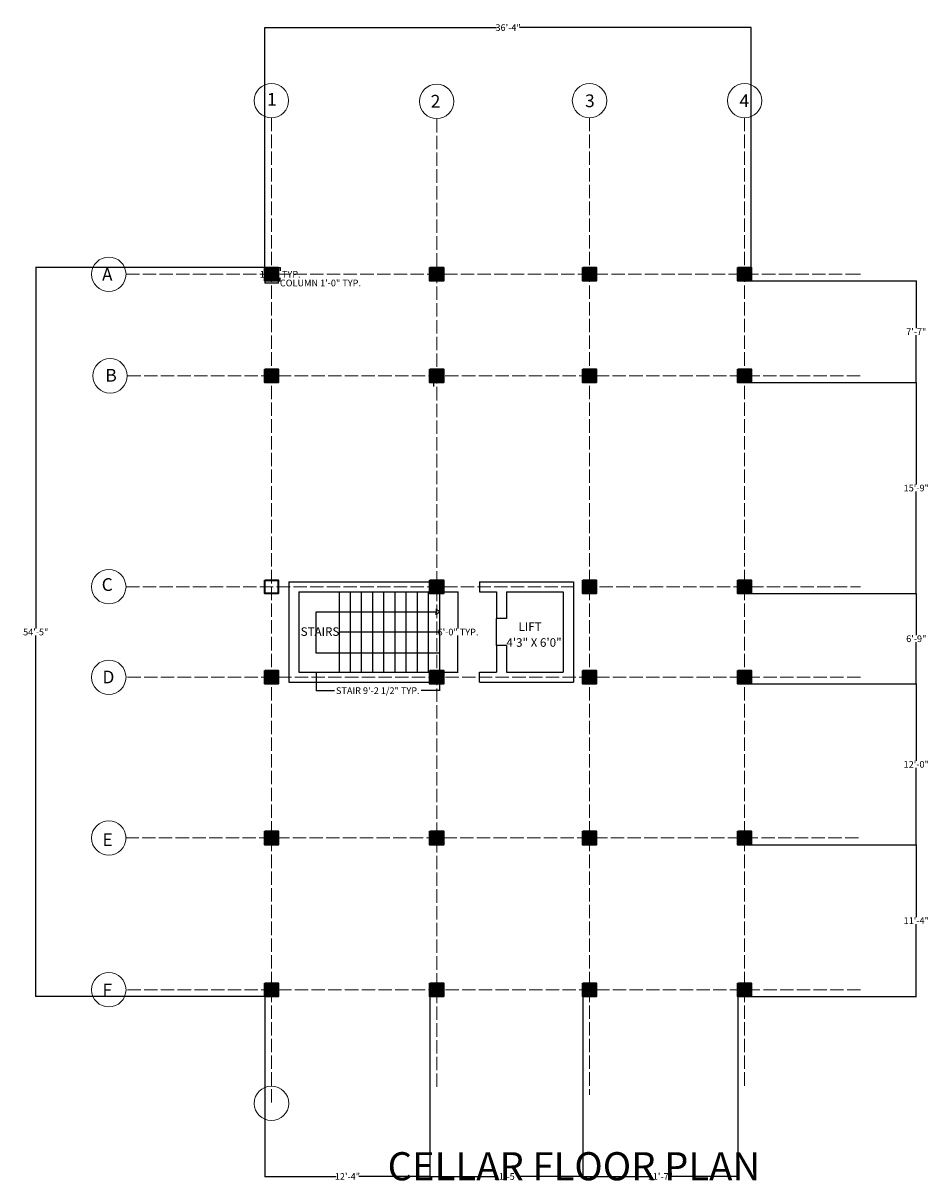
# Model space of a CAD drawing. Units: inches. Extents: x -113 to 5399, y -1393 to 3302.
# Tile 1 of 40: x -113 to 699, y -30 to 1007. Entities that reach past the tile are written whole.
import ezdxf

# ---------------------------------------------------------------- set-up
doc = ezdxf.new("R2010")
doc.units = ezdxf.units.IN
doc.header["$MEASUREMENT"] = 0
doc.linetypes.add('ACAD_ISO02W100', pattern=[15, 12, -3])
for name, color, linetype, lineweight in [('A-ANNO-DIMS', 254, 'Continuous', 18), ('A-ANNO-TEXT', 7, 'Continuous', 25), ('A-AREA-IDEN', 4, 'Continuous', 18), ('A-COLS', 7, 'Continuous', 35), ('A-GRID-IDEN', 7, 'Continuous', 18), ('GRIDS', 7, 'ACAD_ISO02W100', 13), ('stairs', 210, 'Continuous', 25), ('walls', 1, 'Continuous', 25)]:
    doc.layers.add(name, color=color, linetype=linetype, lineweight=lineweight)
doc.styles.get("Standard").update_dxf_attribs({"font": 'arial.ttf'})
doc.dimstyles.get("Standard").update_dxf_attribs({"dimtxt": 6, "dimasz": 0.18, "dimexe": 0.18, "dimexo": 0.0625, "dimgap": 0.09, "dimtad": 0, "dimtih": 1, "dimtoh": 1, "dimdec": 1, "dimzin": 0, "dimdsep": 46, "dimlunit": 4, "dimtxsty": 'Standard', "dimblk": 'ARCHTICK', "dimcen": 0.09, "dimadec": 0, "dimazin": 0, "dimtfac": 1, "dimtdec": 1, "dimtofl": 0, "dimtmove": 0, "dimatfit": 3, "dimfxl": 1, "dimtolj": 1, "dimtzin": 0, "dimarcsym": 0})

# ---------------------------------------------------------------- blocks, each defined once
blk = doc.blocks.new('COLUMN-12IN-SQUARE')
h = blk.add_hatch(color=256)
h.dxf.hatch_style = 1
h.paths.add_polyline_path([(6, 6), (-6, 6), (-6, -6), (6, -6)])
blk.add_lwpolyline([(-6, 6), (6, 6), (6, -6), (-6, -6)], close=True)
blk = doc.blocks.new('STAIR-CELLAR-PLAN')
for p, q in [((20.5, 72), (20.5, 0)), ((30.5, 72), (30.5, 0)), ((40.5, 72), (40.5, 0)), ((50.5, 72), (50.5, 0)), ((60.5, 72), (60.5, 0)), ((70.5, 72), (70.5, 0)), ((80.5, 72), (80.5, 0)), ((90.5, 72), (90.5, 0)), ((100.5, 72), (100.5, 0)), ((110.5, 70.5), (110.5, 1.5)), ((0, 17.1), (0, 54.1)), ((0, 54.1), (107.6, 54.1)), ((110.5, 54.1), (107.6, 56.9)), ((107.6, 56.9), (107.6, 54.1)), ((110.5, 54.1), (107.6, 51.4)), ((107.6, 51.4), (107.6, 54.1)), ((110.5, 36), (20.5, 36)), ((110.5, 17.1), (0, 17.1))]:
    blk.add_line(p, q)
blk = doc.blocks.new('GRID-BUBBLE-A')
blk.add_circle((0, 0), 15.4)
blk.add_text('A', height=11.4).set_placement((-6.1, -5.9))
blk = doc.blocks.new('GRID-BUBBLE-B')
blk.add_circle((0, 0), 15.4)
blk.add_text('B', height=11.4).set_placement((-4.2, -5.2))
blk = doc.blocks.new('GRID-BUBBLE-C')
blk.add_circle((0, 0), 15.4)
blk.add_text('C', height=11.4).set_placement((-6.4, -3.7))
blk = doc.blocks.new('GRID-BUBBLE-D')
blk.add_circle((0, 0), 15.4)
blk.add_text('D', height=11.4).set_placement((-5.7, -5.5))
blk = doc.blocks.new('GRID-BUBBLE-E')
blk.add_circle((0, 0), 15.4)
blk.add_text('E', height=11.4).set_placement((-5.7, -7.1))
blk = doc.blocks.new('GRID-BUBBLE-F')
blk.add_circle((0, 0), 15.4)
blk.add_text('F', height=11.4).set_placement((-5.7, -5.8))
blk = doc.blocks.new('GRID-BUBBLE-1')
blk.add_circle((0, 0), 15.4)
blk.add_text('1', height=11.4).set_placement((-4, -4.5))
blk = doc.blocks.new('GRID-BUBBLE-2')
blk.add_circle((0, 0), 15.4)
blk.add_text('2', height=11.4).set_placement((-5.3, -5.5))
blk = doc.blocks.new('GRID-BUBBLE-3')
blk.add_circle((0, 0), 15.4)
blk.add_text('3', height=11.4).set_placement((-4, -5.8))
blk = doc.blocks.new('GRID-BUBBLE-4')
blk.add_circle((0, 0), 15.4)
blk.add_text('4', height=11.4).set_placement((-4.6, -5.8))
blk = doc.blocks.new('_ArchTick')
at = {"color": 0, "linetype": 'ByBlock', "const_width": 0.15}
blk.add_lwpolyline([(-0.5, -0.5), (0.5, 0.5)], dxfattribs=at)
blk = doc.blocks.new('*D169')
at = {"layer": 'A-ANNO-DIMS', "color": 0, "lineweight": -2, "transparency": 16777216}
for p, q in [((103.6, 776), (103.6, 774.1)), ((103.6, 774.2), (115.6, 774.2)), ((115.6, 776), (115.6, 774.1)), ((115.6, 774.2), (115.8, 774.2))]:
    blk.add_line(p, q, dxfattribs=at)
at = {"layer": 'Defpoints', "color": 0, "transparency": 16777216}
for p in [(103.6, 776), (115.6, 776), (115.6, 774.2)]:
    blk.add_point(p, dxfattribs=at)
at = {"layer": 'A-ANNO-DIMS', "color": 0, "lineweight": -2, "transparency": 16777216, "xscale": 0.18, "yscale": 0.18, "zscale": 0.18, "rotation": 180}
blk.add_blockref('_ArchTick', (103.6, 774.2), dxfattribs=at)
at = {"layer": 'A-ANNO-DIMS', "color": 0, "lineweight": -2, "transparency": 16777216, "xscale": 0.18, "yscale": 0.18, "zscale": 0.18}
blk.add_blockref('_ArchTick', (115.6, 774.2), dxfattribs=at)
at = {"layer": 'A-ANNO-DIMS', "color": 0, "transparency": 16777216, "insert": (153.5, 774.2), "char_height": 6, "attachment_point": 5}
blk.add_mtext('\\A1;COLUMN 1\'-0" TYP.', dxfattribs=at)
blk = doc.blocks.new('*D170')
at = {"layer": 'A-ANNO-DIMS', "color": 0, "lineweight": -2, "transparency": 16777216}
for p, q in [((115.7, 788), (117.6, 788)), ((117.4, 788), (117.4, 785.2)), ((117.4, 776), (117.4, 778.9)), ((115.7, 776), (117.6, 776))]:
    blk.add_line(p, q, dxfattribs=at)
at = {"layer": 'Defpoints', "color": 0, "transparency": 16777216}
for p in [(115.6, 788), (117.4, 788), (115.6, 776)]:
    blk.add_point(p, dxfattribs=at)
at = {"layer": 'A-ANNO-DIMS', "color": 0, "lineweight": -2, "transparency": 16777216, "xscale": 0.18, "yscale": 0.18, "zscale": 0.18}
for p, rotation in [((117.4, 788), 90), ((117.4, 776), 270)]:
    blk.add_blockref('_ArchTick', p, dxfattribs=dict(at, rotation=rotation))
at = {"layer": 'A-ANNO-DIMS', "color": 0, "transparency": 16777216, "insert": (117.4, 782), "char_height": 6, "attachment_point": 5}
blk.add_mtext('\\A1;1\'-0" TYP.', dxfattribs=at)
blk = doc.blocks.new('*D195')
at = {"layer": 'A-ANNO-DIMS', "color": 0, "lineweight": -2, "transparency": 16777216}
for p, q in [((149.7, 425.5), (149.7, 408.8)), ((260.2, 425.5), (260.2, 408.8)), ((149.7, 409), (166.1, 409)), ((260.2, 409), (243.8, 409))]:
    blk.add_line(p, q, dxfattribs=at)
at = {"layer": 'Defpoints', "color": 0, "transparency": 16777216}
for p in [(149.7, 425.5), (260.2, 425.5), (260.2, 409)]:
    blk.add_point(p, dxfattribs=at)
at = {"layer": 'A-ANNO-DIMS', "color": 0, "lineweight": -2, "transparency": 16777216, "xscale": 0.18, "yscale": 0.18, "zscale": 0.18, "rotation": 180}
blk.add_blockref('_ArchTick', (149.7, 409), dxfattribs=at)
at = {"layer": 'A-ANNO-DIMS', "color": 0, "lineweight": -2, "transparency": 16777216, "xscale": 0.18, "yscale": 0.18, "zscale": 0.18}
blk.add_blockref('_ArchTick', (260.2, 409), dxfattribs=at)
at = {"layer": 'A-ANNO-DIMS', "color": 0, "transparency": 16777216, "insert": (204.9, 409), "char_height": 6, "attachment_point": 5}
blk.add_mtext('\\A1;STAIR 9\'-2 1/2" TYP.', dxfattribs=at)
blk = doc.blocks.new('*D196')
at = {"layer": 'A-ANNO-DIMS', "color": 0, "lineweight": -2, "transparency": 16777216}
for p, q in [((260.3, 497.5), (277, 497.5)), ((276.8, 497.5), (276.8, 464.7)), ((276.8, 425.5), (276.8, 458.4)), ((260.3, 425.5), (277, 425.5))]:
    blk.add_line(p, q, dxfattribs=at)
at = {"layer": 'Defpoints', "color": 0, "transparency": 16777216}
for p in [(260.2, 497.5), (276.8, 497.5), (260.2, 425.5)]:
    blk.add_point(p, dxfattribs=at)
at = {"layer": 'A-ANNO-DIMS', "color": 0, "lineweight": -2, "transparency": 16777216, "xscale": 0.18, "yscale": 0.18, "zscale": 0.18}
for p, rotation in [((276.8, 497.5), 90), ((276.8, 425.5), 270)]:
    blk.add_blockref('_ArchTick', p, dxfattribs=dict(at, rotation=rotation))
at = {"layer": 'A-ANNO-DIMS', "color": 0, "transparency": 16777216, "insert": (276.8, 461.5), "char_height": 6, "attachment_point": 5}
blk.add_mtext('\\A1;6\'-0" TYP.', dxfattribs=at)
blk = doc.blocks.new('*D197')
at = {"layer": 'A-ANNO-DIMS', "color": 0, "lineweight": -2, "transparency": 16777216}
for p, q in [((103.6, 788.1), (103.6, 1003.2)), ((103.6, 1003), (311.3, 1003)), ((539.7, 1003), (332, 1003)), ((539.7, 788.1), (539.7, 1003.2))]:
    blk.add_line(p, q, dxfattribs=at)
at = {"layer": 'Defpoints', "color": 0, "transparency": 16777216}
for p in [(539.7, 1003), (103.6, 788), (539.7, 788)]:
    blk.add_point(p, dxfattribs=at)
at = {"layer": 'A-ANNO-DIMS', "color": 0, "lineweight": -2, "transparency": 16777216, "xscale": 0.18, "yscale": 0.18, "zscale": 0.18, "rotation": 180}
blk.add_blockref('_ArchTick', (103.6, 1003), dxfattribs=at)
at = {"layer": 'A-ANNO-DIMS', "color": 0, "lineweight": -2, "transparency": 16777216, "xscale": 0.18, "yscale": 0.18, "zscale": 0.18}
blk.add_blockref('_ArchTick', (539.7, 1003), dxfattribs=at)
at = {"layer": 'A-ANNO-DIMS', "color": 0, "transparency": 16777216, "insert": (321.7, 1003), "char_height": 6, "attachment_point": 5}
blk.add_mtext('\\A1;36\'-4"', dxfattribs=at)
blk = doc.blocks.new('*D198')
at = {"layer": 'A-ANNO-DIMS', "color": 0, "lineweight": -2, "transparency": 16777216}
for p, q in [((103.6, 788), (-101.8, 788)), ((-101.7, 788), (-101.7, 464.7)), ((-101.7, 135), (-101.7, 458.4)), ((103.6, 135), (-101.8, 135))]:
    blk.add_line(p, q, dxfattribs=at)
at = {"layer": 'Defpoints', "color": 0, "transparency": 16777216}
for p in [(-101.7, 788), (103.6, 788), (103.6, 135)]:
    blk.add_point(p, dxfattribs=at)
at = {"layer": 'A-ANNO-DIMS', "color": 0, "lineweight": -2, "transparency": 16777216, "xscale": 0.18, "yscale": 0.18, "zscale": 0.18}
for p, rotation in [((-101.7, 788), 90), ((-101.7, 135), 270)]:
    blk.add_blockref('_ArchTick', p, dxfattribs=dict(at, rotation=rotation))
at = {"layer": 'A-ANNO-DIMS', "color": 0, "transparency": 16777216, "insert": (-101.7, 461.5), "char_height": 6, "attachment_point": 5}
blk.add_mtext('\\A1;54\'-5"', dxfattribs=at)
blk = doc.blocks.new('*D199')
at = {"layer": 'A-ANNO-DIMS', "color": 0, "lineweight": -2, "transparency": 16777216}
for p, q in [((103.6, 135), (103.6, -26.4)), ((251.7, 135), (251.7, -26.4)), ((103.6, -26.2), (167.5, -26.2)), ((251.7, -26.2), (187.8, -26.2))]:
    blk.add_line(p, q, dxfattribs=at)
at = {"layer": 'Defpoints', "color": 0, "transparency": 16777216}
for p in [(103.6, 135), (251.7, 135), (251.7, -26.2)]:
    blk.add_point(p, dxfattribs=at)
at = {"layer": 'A-ANNO-DIMS', "color": 0, "lineweight": -2, "transparency": 16777216, "xscale": 0.18, "yscale": 0.18, "zscale": 0.18, "rotation": 180}
blk.add_blockref('_ArchTick', (103.6, -26.2), dxfattribs=at)
at = {"layer": 'A-ANNO-DIMS', "color": 0, "lineweight": -2, "transparency": 16777216, "xscale": 0.18, "yscale": 0.18, "zscale": 0.18}
blk.add_blockref('_ArchTick', (251.7, -26.2), dxfattribs=at)
at = {"layer": 'A-ANNO-DIMS', "color": 0, "transparency": 16777216, "insert": (177.7, -26.2), "char_height": 6, "attachment_point": 5}
blk.add_mtext('\\A1;12\'-4"', dxfattribs=at)
blk = doc.blocks.new('*D200')
at = {"layer": 'A-ANNO-DIMS', "color": 0, "lineweight": -2, "transparency": 16777216}
for p, q in [((251.7, 135), (251.7, -26.4)), ((388.7, 135), (388.7, -26.4)), ((251.7, -26.2), (310.1, -26.2)), ((388.7, -26.2), (330.3, -26.2))]:
    blk.add_line(p, q, dxfattribs=at)
at = {"layer": 'Defpoints', "color": 0, "transparency": 16777216}
for p in [(251.7, 135), (388.7, 135), (388.7, -26.2)]:
    blk.add_point(p, dxfattribs=at)
at = {"layer": 'A-ANNO-DIMS', "color": 0, "lineweight": -2, "transparency": 16777216, "xscale": 0.18, "yscale": 0.18, "zscale": 0.18, "rotation": 180}
blk.add_blockref('_ArchTick', (251.7, -26.2), dxfattribs=at)
at = {"layer": 'A-ANNO-DIMS', "color": 0, "lineweight": -2, "transparency": 16777216, "xscale": 0.18, "yscale": 0.18, "zscale": 0.18}
blk.add_blockref('_ArchTick', (388.7, -26.2), dxfattribs=at)
at = {"layer": 'A-ANNO-DIMS', "color": 0, "transparency": 16777216, "insert": (320.2, -26.2), "char_height": 6, "attachment_point": 5}
blk.add_mtext('\\A1;11\'-5"', dxfattribs=at)
blk = doc.blocks.new('*D201')
at = {"layer": 'A-ANNO-DIMS', "color": 0, "lineweight": -2, "transparency": 16777216}
for p, q in [((388.7, 135), (388.7, -26.4)), ((527.7, 135), (527.7, -26.4)), ((388.7, -26.2), (448.1, -26.2)), ((527.7, -26.2), (468.3, -26.2))]:
    blk.add_line(p, q, dxfattribs=at)
at = {"layer": 'Defpoints', "color": 0, "transparency": 16777216}
for p in [(388.7, 135), (527.7, 135), (527.7, -26.2)]:
    blk.add_point(p, dxfattribs=at)
at = {"layer": 'A-ANNO-DIMS', "color": 0, "lineweight": -2, "transparency": 16777216, "xscale": 0.18, "yscale": 0.18, "zscale": 0.18, "rotation": 180}
blk.add_blockref('_ArchTick', (388.7, -26.2), dxfattribs=at)
at = {"layer": 'A-ANNO-DIMS', "color": 0, "lineweight": -2, "transparency": 16777216, "xscale": 0.18, "yscale": 0.18, "zscale": 0.18}
blk.add_blockref('_ArchTick', (527.7, -26.2), dxfattribs=at)
at = {"layer": 'A-ANNO-DIMS', "color": 0, "transparency": 16777216, "insert": (458.2, -26.2), "char_height": 6, "attachment_point": 5}
blk.add_mtext('\\A1;11\'-7"', dxfattribs=at)
blk = doc.blocks.new('*D202')
at = {"layer": 'A-ANNO-DIMS', "color": 0, "lineweight": -2, "transparency": 16777216}
for p, q in [((539.8, 271), (687.7, 271)), ((687.6, 271), (687.6, 206.1)), ((687.6, 135), (687.6, 199.9)), ((539.8, 135), (687.7, 135))]:
    blk.add_line(p, q, dxfattribs=at)
at = {"layer": 'Defpoints', "color": 0, "transparency": 16777216}
for p in [(539.7, 271), (687.6, 271), (539.7, 135)]:
    blk.add_point(p, dxfattribs=at)
at = {"layer": 'A-ANNO-DIMS', "color": 0, "lineweight": -2, "transparency": 16777216, "xscale": 0.18, "yscale": 0.18, "zscale": 0.18}
for p, rotation in [((687.6, 271), 90), ((687.6, 135), 270)]:
    blk.add_blockref('_ArchTick', p, dxfattribs=dict(at, rotation=rotation))
at = {"layer": 'A-ANNO-DIMS', "color": 0, "transparency": 16777216, "insert": (687.6, 203), "char_height": 6, "attachment_point": 5}
blk.add_mtext('\\A1;11\'-4"', dxfattribs=at)
blk = doc.blocks.new('*D203')
at = {"layer": 'A-ANNO-DIMS', "color": 0, "lineweight": -2, "transparency": 16777216}
for p, q in [((539.8, 415), (687.7, 415)), ((687.6, 415), (687.6, 346.2)), ((687.6, 271), (687.6, 339.9)), ((539.8, 271), (687.7, 271))]:
    blk.add_line(p, q, dxfattribs=at)
at = {"layer": 'Defpoints', "color": 0, "transparency": 16777216}
for p in [(539.7, 415), (687.6, 415), (539.7, 271)]:
    blk.add_point(p, dxfattribs=at)
at = {"layer": 'A-ANNO-DIMS', "color": 0, "lineweight": -2, "transparency": 16777216, "xscale": 0.18, "yscale": 0.18, "zscale": 0.18}
for p, rotation in [((687.6, 415), 90), ((687.6, 271), 270)]:
    blk.add_blockref('_ArchTick', p, dxfattribs=dict(at, rotation=rotation))
at = {"layer": 'A-ANNO-DIMS', "color": 0, "transparency": 16777216, "insert": (687.6, 343), "char_height": 6, "attachment_point": 5}
blk.add_mtext('\\A1;12\'-0"', dxfattribs=at)
blk = doc.blocks.new('*D204')
at = {"layer": 'A-ANNO-DIMS', "color": 0, "lineweight": -2, "transparency": 16777216}
for p, q in [((539.8, 496), (687.7, 496)), ((687.6, 496), (687.6, 458.7)), ((687.6, 415), (687.6, 452.4)), ((539.8, 415), (687.7, 415))]:
    blk.add_line(p, q, dxfattribs=at)
at = {"layer": 'Defpoints', "color": 0, "transparency": 16777216}
for p in [(539.7, 496), (687.6, 496), (539.7, 415)]:
    blk.add_point(p, dxfattribs=at)
at = {"layer": 'A-ANNO-DIMS', "color": 0, "lineweight": -2, "transparency": 16777216, "xscale": 0.18, "yscale": 0.18, "zscale": 0.18}
for p, rotation in [((687.6, 496), 90), ((687.6, 415), 270)]:
    blk.add_blockref('_ArchTick', p, dxfattribs=dict(at, rotation=rotation))
at = {"layer": 'A-ANNO-DIMS', "color": 0, "transparency": 16777216, "insert": (687.6, 455.5), "char_height": 6, "attachment_point": 5}
blk.add_mtext('\\A1;6\'-9"', dxfattribs=at)
blk = doc.blocks.new('*D205')
at = {"layer": 'A-ANNO-DIMS', "color": 0, "lineweight": -2, "transparency": 16777216}
for p, q in [((539.8, 685), (687.7, 685)), ((687.6, 685), (687.6, 593.7)), ((687.6, 496), (687.6, 587.4)), ((539.8, 496), (687.7, 496))]:
    blk.add_line(p, q, dxfattribs=at)
at = {"layer": 'Defpoints', "color": 0, "transparency": 16777216}
for p in [(539.7, 685), (687.6, 685), (539.7, 496)]:
    blk.add_point(p, dxfattribs=at)
at = {"layer": 'A-ANNO-DIMS', "color": 0, "lineweight": -2, "transparency": 16777216, "xscale": 0.18, "yscale": 0.18, "zscale": 0.18}
for p, rotation in [((687.6, 685), 90), ((687.6, 496), 270)]:
    blk.add_blockref('_ArchTick', p, dxfattribs=dict(at, rotation=rotation))
at = {"layer": 'A-ANNO-DIMS', "color": 0, "transparency": 16777216, "insert": (687.6, 590.5), "char_height": 6, "attachment_point": 5}
blk.add_mtext('\\A1;15\'-9"', dxfattribs=at)
blk = doc.blocks.new('*D206')
at = {"layer": 'A-ANNO-DIMS', "color": 0, "lineweight": -2, "transparency": 16777216}
for p, q in [((539.753481, 776.031978), (687.733268, 776.031978)), ((687.553268, 776.031978), (687.553268, 733.621978)), ((687.553268, 685.031978), (687.553268, 727.441978)), ((539.753481, 685.031978), (687.733268, 685.031978))]:
    blk.add_line(p, q, dxfattribs=at)
at = {"layer": 'Defpoints', "color": 0, "transparency": 16777216}
for p in [(539.690981, 776.031978), (687.553268, 776.031978), (539.690981, 685.031978)]:
    blk.add_point(p, dxfattribs=at)
at = {"layer": 'A-ANNO-DIMS', "color": 0, "lineweight": -2, "transparency": 16777216, "xscale": 0.18, "yscale": 0.18, "zscale": 0.18}
for p, rotation in [((687.553268, 776.031978), 90), ((687.553268, 685.031978), 270)]:
    blk.add_blockref('_ArchTick', p, dxfattribs=dict(at, rotation=rotation))
at = {"layer": 'A-ANNO-DIMS', "color": 0, "transparency": 16777216, "insert": (687.553268, 730.531978), "char_height": 6, "attachment_point": 5}
blk.add_mtext('\\A1;7\'-7"', dxfattribs=at)

msp = doc.modelspace()

# ---------------------------------------------------------------- linework, layer by layer
at = {"layer": 'A-COLS'}
msp.add_lwpolyline([(103.61, 508.03), (115.61, 508.03), (115.61, 496.03), (103.61, 496.03)], close=True, dxfattribs=at)
at = {"layer": 'A-GRID-IDEN'}
msp.add_circle((109.61, 39.31), 15.44, dxfattribs=at)
at = {"layer": 'GRIDS'}
for p, q in [((109.61, 922.09), (109.61, 39.31)), ((257.69, 54.04), (257.69, 921.39)), ((394.69, 922.09), (394.69, 46.81)), ((533.69, 922.09), (533.69, 54.5)), ((-20.74, 782.03), (628.14, 782.03)), ((628.14, 782.03), (637.5, 782.03)), ((-19.62, 691.03), (637.5, 691.03)), ((-20.74, 502.03), (380.19, 502.03)), ((388.69, 502.03), (637.5, 502.03)), ((637.5, 421.03), (-20.74, 421.03)), ((-21.29, 277.03), (637.5, 277.03)), ((637.5, 141.03), (-20.74, 141.03))]:
    msp.add_line(p, q, dxfattribs=at)
at = {"layer": 'walls'}
for p, q in [((255.19, 681.53), (255.19, 693.53)), ((255.19, 693.53), (260.19, 693.53)), ((125.19, 506.53), (125.19, 416.53)), ((125.19, 506.53), (251.69, 506.53)), ((260.19, 506.53), (260.19, 497.53)), ((296.19, 506.53), (380.19, 506.53)), ((296.19, 506.53), (296.19, 497.53)), ((380.19, 506.53), (380.19, 425.53)), ((388.69, 506.53), (392.19, 506.53)), ((134.19, 497.53), (251.69, 497.53)), ((134.19, 497.53), (134.19, 425.53)), ((296.19, 497.53), (311.19, 497.53)), ((311.19, 497.53), (311.19, 473.53)), ((320.19, 497.53), (320.19, 473.53)), ((320.19, 497.53), (371.19, 497.53)), ((371.19, 497.53), (371.19, 425.53)), ((388.69, 497.53), (397.19, 497.53)), ((320.19, 473.53), (311.19, 473.53)), ((311.19, 449.53), (311.19, 473.53)), ((380.19, 457.03), (380.19, 416.53)), ((311.19, 449.53), (311.19, 425.53)), ((320.19, 449.53), (311.19, 449.53)), ((320.19, 449.53), (320.19, 425.53)), ((134.19, 425.53), (251.69, 425.53)), ((260.19, 416.53), (260.19, 425.53)), ((296.19, 425.53), (311.19, 425.53)), ((296.19, 416.53), (296.19, 425.53)), ((320.19, 425.53), (371.19, 425.53)), ((388.69, 425.53), (397.19, 425.53)), ((125.19, 416.53), (251.69, 416.53)), ((296.19, 416.53), (380.19, 416.53)), ((388.69, 416.53), (392.19, 416.53)), ((255.19, 274.53), (260.19, 274.53))]:
    msp.add_line(p, q, dxfattribs=at)

# ---------------------------------------------------------------- block references
at = {"layer": 'A-COLS'}
for p in [(109.61, 782.03), (257.69, 782.03), (394.69, 782.03), (533.69, 782.03), (109.61, 691.03), (257.69, 691.03), (394.69, 691.03), (533.69, 691.03), (257.69, 502.03), (394.69, 502.03), (533.69, 502.03), (109.61, 421.03), (257.69, 421.03), (394.69, 421.03), (533.69, 421.03), (109.61, 277.03), (257.69, 277.03), (394.69, 277.03), (533.69, 277.03), (109.61, 141.03), (257.69, 141.03), (394.69, 141.03), (533.69, 141.03)]:
    msp.add_blockref('COLUMN-12IN-SQUARE', p, dxfattribs=at)
at = {"layer": 'A-GRID-IDEN'}
for name, p in [('GRID-BUBBLE-1', (109.61, 937.53)), ('GRID-BUBBLE-2', (257.69, 936.83)), ('GRID-BUBBLE-3', (394.69, 937.53)), ('GRID-BUBBLE-4', (533.69, 937.53)), ('GRID-BUBBLE-A', (-36.18, 782.03)), ('GRID-BUBBLE-B', (-35.06, 691.03)), ('GRID-BUBBLE-C', (-36.18, 502.03)), ('GRID-BUBBLE-D', (-36.18, 421.03)), ('GRID-BUBBLE-E', (-36.18, 277.03)), ('GRID-BUBBLE-F', (-36.18, 141.03))]:
    msp.add_blockref(name, p, dxfattribs=at)
at = {"layer": 'stairs'}
msp.add_blockref('STAIR-CELLAR-PLAN', (149.65, 425.53), dxfattribs=at)

# ---------------------------------------------------------------- texts
at = {"layer": 'A-ANNO-TEXT'}
msp.add_text('CELLAR FLOOR PLAN', height=25.17, dxfattribs=at).set_placement((213.7, -29.6))
at = {"layer": 'A-AREA-IDEN'}
for s, height, p in [('LIFT', 7.647, (331.08, 462.59)), ('STAIRS', 7.647, (135.74, 458.09)), ('4\'3" X 6\'0"', 7.6473, (320.19, 448.32))]:
    msp.add_text(s, height=height, dxfattribs=at).set_placement(p)

# ---------------------------------------------------------------- dimensions: what is measured, and where the dimension line sits
at = {"layer": 'A-ANNO-DIMS'}
for base, p1, p2, picture, middle in [((539.69, 1003.02), (103.61, 788.03), (539.69, 788.03), '*D197', (321.65, 1003.02)), ((251.69, -26.18), (103.61, 135.03), (251.69, 135.03), '*D199', (177.65, -26.18)), ((388.69, -26.18), (251.69, 135.03), (388.69, 135.03), '*D200', (320.19, -26.18)), ((527.69, -26.18), (388.69, 135.03), (527.69, 135.03), '*D201', (458.19, -26.18))]:
    dim = msp.add_linear_dim(base=base, p1=p1, p2=p2, dimstyle='Standard', override={"dimdec": 1, "dimlfac": 1, "dimrnd": 0, "dimzin": 1, "dimdsep": 46, "dimlunit": 4, "dimfrac": 2}, dxfattribs=at)
    dim.commit()
    dim.dimension.update_dxf_attribs({"geometry": picture, "text_midpoint": middle})
for base, p1, p2, picture, middle in [((117.41, 788.03), (115.61, 776.03), (115.61, 788.03), '*D170', (117.41, 782.03)), ((276.77, 497.53), (260.19, 425.53), (260.19, 497.53), '*D196', (276.77, 461.53))]:
    dim = msp.add_linear_dim(base=base, p1=p1, p2=p2, angle=90, text='<> TYP.', dimstyle='Standard', override={"dimdec": 1, "dimlfac": 1, "dimrnd": 0, "dimzin": 1, "dimdsep": 46, "dimlunit": 4, "dimfrac": 2}, dxfattribs=at)
    dim.commit()
    dim.dimension.update_dxf_attribs({"geometry": picture, "text_midpoint": middle})
for base, p1, p2, text, picture, middle in [((115.61, 774.23), (103.61, 776.03), (115.61, 776.03), 'COLUMN <> TYP.', '*D169', (153.46, 774.23)), ((260.19, 408.95), (149.65, 425.53), (260.19, 425.53), 'STAIR <> TYP.', '*D195', (204.92, 408.95))]:
    dim = msp.add_linear_dim(base=base, p1=p1, p2=p2, text=text, dimstyle='Standard', override={"dimdec": 1, "dimlfac": 1, "dimrnd": 0, "dimzin": 1, "dimdsep": 46, "dimlunit": 4, "dimfrac": 2}, dxfattribs=at)
    dim.commit()
    dim.dimension.update_dxf_attribs({"geometry": picture, "text_midpoint": middle})
for base, p1, p2, picture, middle in [((-101.67, 788.03), (103.61, 135.03), (103.61, 788.03), '*D198', (-101.67, 461.53)), ((687.55, 776.03), (539.69, 685.03), (539.69, 776.03), '*D206', (687.55, 730.53)), ((687.55, 685.03), (539.69, 496.03), (539.69, 685.03), '*D205', (687.55, 590.53)), ((687.55, 496.03), (539.69, 415.03), (539.69, 496.03), '*D204', (687.55, 455.53)), ((687.55, 415.03), (539.69, 271.03), (539.69, 415.03), '*D203', (687.55, 343.03)), ((687.55, 271.03), (539.69, 135.03), (539.69, 271.03), '*D202', (687.55, 203.03))]:
    dim = msp.add_linear_dim(base=base, p1=p1, p2=p2, angle=90, dimstyle='Standard', override={"dimdec": 1, "dimlfac": 1, "dimrnd": 0, "dimzin": 1, "dimdsep": 46, "dimlunit": 4, "dimfrac": 2}, dxfattribs=at)
    dim.commit()
    dim.dimension.update_dxf_attribs({"geometry": picture, "text_midpoint": middle})

doc.saveas('drawing.dxf')
